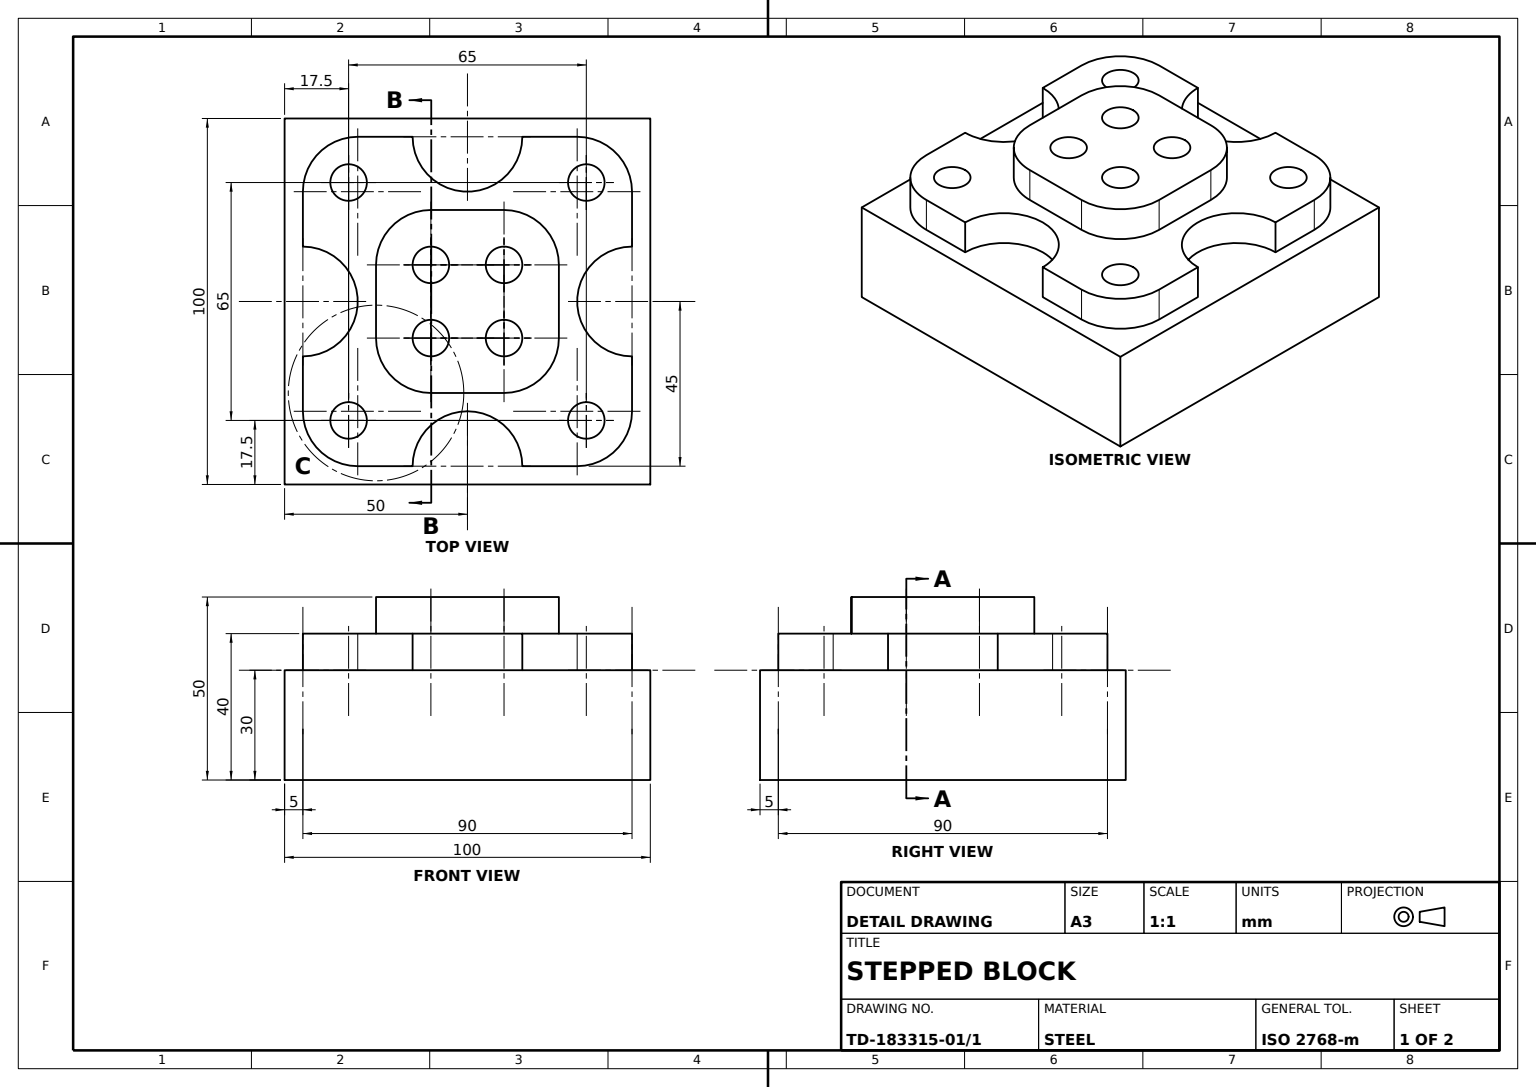
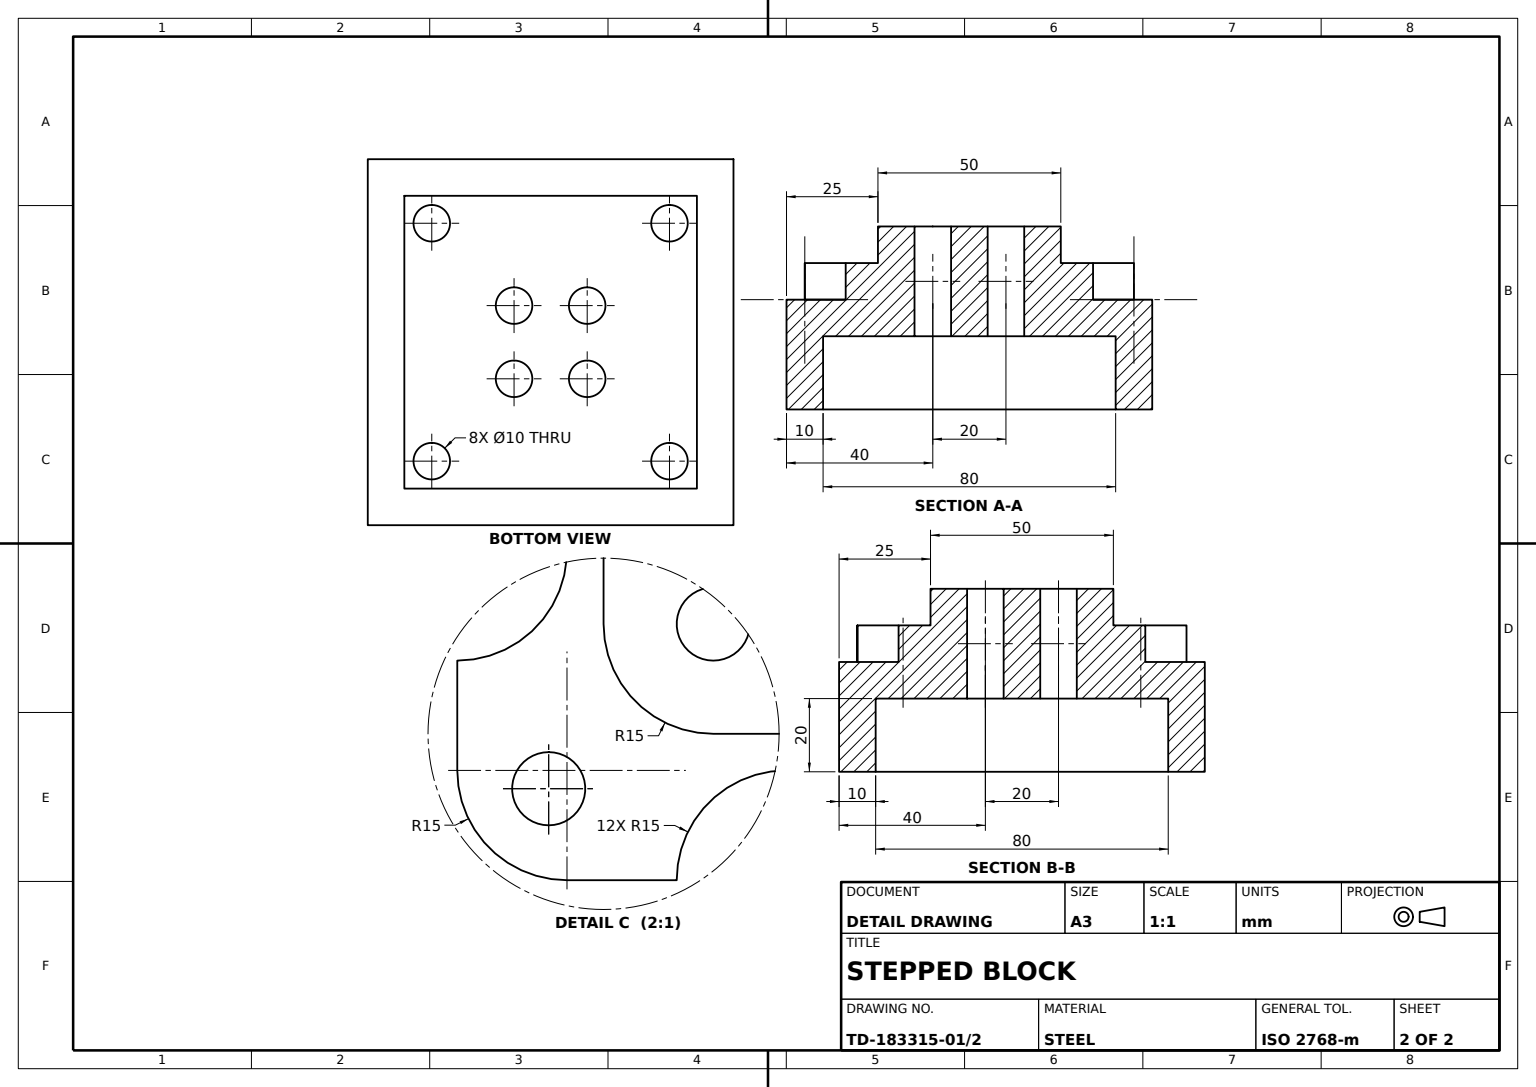
from build123d import *

# Parameters (mm, degrees)
BASE_SQUARE_SKETCH_W        = 100
BASE_SQUARE_SKETCH_H        = 100
BASE_BLOCK_100X100X30_DEPTH = 30
BASE_SHELL_10MM_T           = -10
CROSS_PLATE_SKETCH_R        = 5
CROSS_PLATE_10MM_DEPTH      = 10
PLATE_HOLES_SKETCH_R        = 5
PLATE_ARM_HOLES_4X_DEPTH    = 82.240384046
CENTRE_BOSS_SKETCH_R        = 5
CENTRE_BOSS_10MM_DEPTH      = 10
CENTRE_HOLES_SKETCH_R       = 5
CENTRE_BOSS_HOLES_4X_DEPTH  = 87.602540378


with BuildPart() as part:
    # Base Square Sketch → Base Block 100x100x30 (new body)
    with BuildSketch(Plane(origin=(0, 0, 0), x_dir=(1, 0, 0), z_dir=(0, 1, 0))):
        Rectangle(BASE_SQUARE_SKETCH_W, BASE_SQUARE_SKETCH_H)
    extrude(amount=BASE_BLOCK_100X100X30_DEPTH)

    # Base Shell 10mm
    base_shell_10mm_openings = [part.faces().sort_by_distance(p)[0] for p in [
        (0, 0, 0),
    ]]
    offset(amount=BASE_SHELL_10MM_T, openings=base_shell_10mm_openings, kind=Kind.INTERSECTION)

    # Cross Plate Sketch → Cross Plate 10mm (add)
    with BuildSketch(Plane(origin=(0, 30, 0), x_dir=(1, 0, 0), z_dir=(0, 1, 0))):
        with BuildLine():
            Line((15, 45), (30, 45))
            ThreePointArc((30, 45), (40.606601718, 40.606601718), (45, 30))
            Line((45, 30), (45, 15))
            ThreePointArc((45, 15), (30, 0), (45, -15))
            Line((45, -15), (45, -30))
            ThreePointArc((45, -30), (40.606601718, -40.606601718), (30, -45))
            Line((30, -45), (15, -45))
            ThreePointArc((15, -45), (0, -30), (-15, -45))
            Line((-15, -45), (-30, -45))
            ThreePointArc((-30, -45), (-40.606601718, -40.606601718), (-45, -30))
            Line((-45, -30), (-45, -15))
            ThreePointArc((-45, -15), (-30, 0), (-45, 15))
            Line((-45, 15), (-45, 30))
            ThreePointArc((-45, 30), (-40.606601718, 40.606601718), (-30, 45))
            Line((-30, 45), (-15, 45))
            ThreePointArc((-15, 45), (0, 30), (15, 45))
        make_face()
        with Locations(Location((-32.5, 32.5, 0), (0, 0, 270))):
            Circle(CROSS_PLATE_SKETCH_R, mode=Mode.SUBTRACT)
        with Locations(Location((32.5, 32.5, 0), (0, 0, 270))):
            Circle(CROSS_PLATE_SKETCH_R, mode=Mode.SUBTRACT)
        with Locations(Location((-32.5, -32.5, 0), (0, 0, 270))):
            Circle(CROSS_PLATE_SKETCH_R, mode=Mode.SUBTRACT)
        with Locations(Location((32.5, -32.5, 0), (0, 0, 270))):
            Circle(CROSS_PLATE_SKETCH_R, mode=Mode.SUBTRACT)
    extrude(amount=CROSS_PLATE_10MM_DEPTH)

    # Plate Holes Sketch → Plate Arm Holes 4x (cut, through all)
    with BuildSketch(Plane(origin=(0, 40, 0), x_dir=(1, 0, 0), z_dir=(0, 1, 0))):
        with Locations(Location((-32.5, 32.5, 0), (0, 0, 90))):
            Circle(PLATE_HOLES_SKETCH_R)
        with Locations(Location((32.5, 32.5, 0), (0, 0, 90))):
            Circle(PLATE_HOLES_SKETCH_R)
        with Locations(Location((32.5, -32.5, 0), (0, 0, 90))):
            Circle(PLATE_HOLES_SKETCH_R)
        with Locations(Location((-32.5, -32.5, 0), (0, 0, 90))):
            Circle(PLATE_HOLES_SKETCH_R)
    extrude(amount=-PLATE_ARM_HOLES_4X_DEPTH, mode=Mode.SUBTRACT)

    # Centre Boss Sketch → Centre Boss 10mm (add)
    with BuildSketch(Plane(origin=(0, 40, 0), x_dir=(1, 0, 0), z_dir=(0, 1, 0))):
        with BuildLine():
            Line((-25, 10), (-25, -10))
            ThreePointArc((-25, -10), (-20.606601718, -20.606601718), (-10, -25))
            Line((-10, -25), (10, -25))
            ThreePointArc((10, -25), (20.606601718, -20.606601718), (25, -10))
            Line((25, -10), (25, 10))
            ThreePointArc((25, 10), (20.606601718, 20.606601718), (10, 25))
            Line((10, 25), (-10, 25))
            ThreePointArc((-10, 25), (-20.606601718, 20.606601718), (-25, 10))
        make_face()
        with Locations(Location((-10, 10, 0), (0, 0, 270))):
            Circle(CENTRE_BOSS_SKETCH_R, mode=Mode.SUBTRACT)
        with Locations(Location((10, 10, 0), (0, 0, 270))):
            Circle(CENTRE_BOSS_SKETCH_R, mode=Mode.SUBTRACT)
        with Locations(Location((10, -10, 0), (0, 0, 270))):
            Circle(CENTRE_BOSS_SKETCH_R, mode=Mode.SUBTRACT)
        with Locations(Location((-10, -10, 0), (0, 0, 270))):
            Circle(CENTRE_BOSS_SKETCH_R, mode=Mode.SUBTRACT)
    extrude(amount=CENTRE_BOSS_10MM_DEPTH)

    # Centre Holes Sketch → Centre Boss Holes 4x (cut, through all)
    with BuildSketch(Plane(origin=(0, 50, 0), x_dir=(1, 0, 0), z_dir=(0, 1, 0))):
        with Locations(Location((-10, 10, 0), (0, 0, 90))):
            Circle(CENTRE_HOLES_SKETCH_R)
        with Locations(Location((10, 10, 0), (0, 0, 90))):
            Circle(CENTRE_HOLES_SKETCH_R)
        with Locations(Location((10, -10, 0), (0, 0, 90))):
            Circle(CENTRE_HOLES_SKETCH_R)
        with Locations(Location((-10, -10, 0), (0, 0, 90))):
            Circle(CENTRE_HOLES_SKETCH_R)
    extrude(amount=-CENTRE_BOSS_HOLES_4X_DEPTH, mode=Mode.SUBTRACT)


solid = part.part
